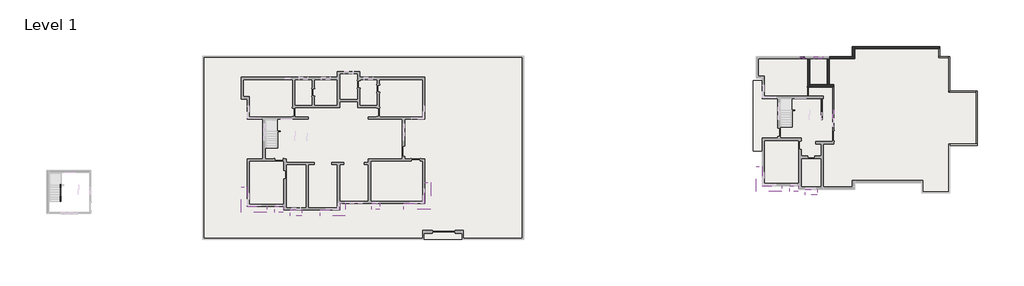
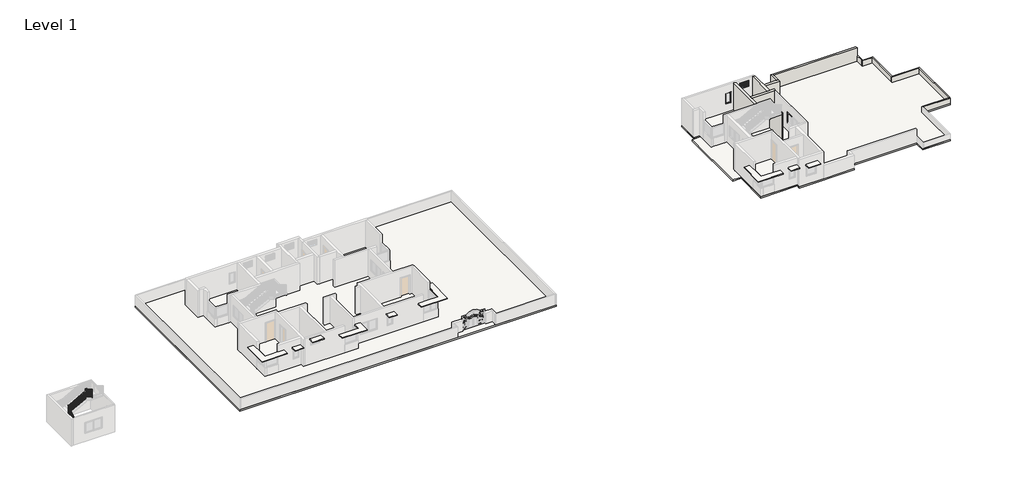
# One storey, part 4 of 9: 13 walls, 11 slabs, 6 members, 1 door, 1 railing, 1 window.
"""IFC4 building model written with IfcOpenShell, lengths in millimetres."""

from ifc_helpers import new_model, si_unit, frame, origin, origin_with_axes, place, context, project, spatial, polyline, outline, extrude, faceted_brep, transform, mapped, element, save
from components import single_flush_door_3_a90ba1ad, member_75074519, member_8d24a278, member_86d06fe4, window_a18e4be4

model = new_model("IFC4")

# Units and contexts
model_context = context("Model", 3, world=origin())
ifc_project = project(units=[si_unit("LENGTHUNIT", "METRE", prefix="MILLI")], contexts=[model_context])

# Site, building, storey
site = spatial("IfcSite", under=ifc_project)
building = spatial("IfcBuilding", under=site)
storey = spatial("IfcBuildingStorey", under=building, Name="Level 1", Elevation=0.0)

# Door
placement = place(None, origin())
single_flush_door_3_shape = single_flush_door_3_a90ba1ad(model_context)
element("IfcDoor", 1, ObjectType="Single-Flush : door 3'", at=placement, inside=storey, context=model_context, shape_type="MappedRepresentation", body=[
    mapped(single_flush_door_3_shape, transform((16302.8100959, 18368.9480703, 0.0), x_axis=(0.0, -1.0, 0.0), y_axis=(1.0, 0.0, 0.0), z_axis=(0.0, 0.0, 1.0))),
])

# Members
member_shape = member_75074519(model_context)
element("IfcMember", 2, ObjectType="Rectangular Mullion : 2.5\" x 5\" rectangular", at=placement, inside=storey, context=model_context, shape_type="MappedRepresentation", body=[
    mapped(member_shape, transform((15959.9100959, 21924.9480703, 914.4), x_axis=(1.0, 0.0, 0.0), y_axis=(0.0, -1.0, 0.0), z_axis=(0.0, 0.0, -1.0))),
])
element("IfcMember", 3, ObjectType="Rectangular Mullion : 2.5\" x 5\" rectangular", at=placement, inside=storey, context=model_context, shape_type="MappedRepresentation", body=[
    mapped(member_shape, transform((15350.3100959, 21924.9480703, 2133.6), x_axis=(-1.0, 0.0, 0.0), y_axis=(0.0, -1.0, 0.0), z_axis=(0.0, 0.0, 1.0))),
])
element("IfcMember", 4, ObjectType="Rectangular Mullion : 2.5\" x 5\" rectangular", at=placement, inside=storey, context=model_context, shape_type="MappedRepresentation", body=[
    mapped(member_shape, transform((18890.1839667, 16463.3540338, 914.4), x_axis=(0.0, 1.0, 0.0), y_axis=(1.0, 0.0, 0.0), z_axis=(0.0, 0.0, -1.0))),
])
member_2_shape = member_8d24a278(model_context)
element("IfcMember", 5, ObjectType="Rectangular Mullion : 2.5\" x 5\" rectangular", at=placement, inside=storey, context=model_context, shape_type="MappedRepresentation", body=[
    mapped(member_2_shape, transform((18890.1839667, 16399.8540338, 2133.6), x_axis=(0.0, 0.0, 1.0), y_axis=(1.0, 0.0, 0.0), z_axis=(0.0, 1.0, 0.0))),
])
member_3_shape = member_86d06fe4(model_context)
element("IfcMember", 6, ObjectType="Rectangular Mullion : 2.5\" x 5\" rectangular", at=placement, inside=storey, context=model_context, shape_type="MappedRepresentation", body=[
    mapped(member_3_shape, transform((15896.4100959, 21924.9480703, 2133.6), x_axis=(0.0, 0.0, 1.0), y_axis=(0.0, -1.0, 0.0), z_axis=(1.0, 0.0, 0.0))),
])
element("IfcMember", 7, ObjectType="Rectangular Mullion : 2.5\" x 5\" rectangular", at=placement, inside=storey, context=model_context, shape_type="MappedRepresentation", body=[
    mapped(member_3_shape, transform((15413.8100959, 21924.9480703, 914.4), x_axis=(0.0, 0.0, -1.0), y_axis=(0.0, -1.0, 0.0), z_axis=(-1.0, 0.0, 0.0))),
])

# Railing
element("IfcRailing", 8, ObjectType="Handrail - Rectangular", at=placement, inside=storey, context=model_context, shape_type="SolidModel", body=[
    faceted_brep([(-62595.4636189, 6754.3199577, 1059.5428571), (-62595.4636189, 6754.3199577, 1001.0339009), (-62544.6636189, 6754.3199577, 1001.0339009), (-62544.6636189, 6754.3199577, 1059.5428571), (-62595.4636189, 8456.1199577, 2032.0), (-62595.4636189, 8506.9199577, 2002.5196152), (-62544.6636189, 8506.9199577, 2002.5196152), (-62544.6636189, 8456.1199577, 2032.0), (-62595.4636189, 8456.1199577, 2261.3257143), (-62595.4636189, 8506.9199577, 2210.5257143), (-62544.6636189, 8506.9199577, 2210.5257143), (-62544.6636189, 8456.1199577, 2261.3257143), (-62595.4636189, 8583.1199577, 2261.3257143), (-62595.4636189, 8583.1199577, 2210.5257143), (-62544.6636189, 8532.3199577, 2210.5257143), (-62544.6636189, 8532.3199577, 2261.3257143), (-62468.4636189, 8583.1199577, 2261.3257143), (-62455.7636189, 8583.1199577, 2210.5257143), (-62455.7636189, 8532.3199577, 2210.5257143), (-62468.4636189, 8532.3199577, 2261.3257143), (-60715.8636189, 8583.1199577, 3196.0457143), (-60665.0636189, 8583.1199577, 3165.5657143), (-60665.0636189, 8532.3199577, 3165.5657143), (-60715.8636189, 8532.3199577, 3196.0457143), (-60715.8636189, 8583.1199577, 3425.3714286), (-60665.0636189, 8583.1199577, 3374.5714286), (-60665.0636189, 8532.3199577, 3374.5714286), (-60715.8636189, 8532.3199577, 3425.3714286), (-60588.8636189, 8583.1199577, 3425.3714286), (-60588.8636189, 8583.1199577, 3374.5714286), (-60639.6636189, 8532.3199577, 3374.5714286), (-60639.6636189, 8532.3199577, 3425.3714286), (-60588.8636189, 8456.1199577, 3425.3714286), (-60588.8636189, 8442.6292843, 3374.5714286), (-60639.6636189, 8442.6292843, 3374.5714286), (-60639.6636189, 8456.1199577, 3425.3714286), (-60588.8636189, 7516.3199577, 3962.4), (-60639.6636189, 7516.3199577, 3962.4), (-60639.6636189, 7516.3199577, 3903.8910438), (-60588.8636189, 7516.3199577, 3903.8910438)], [[[0, 1, 2, 3]], [[1, 0, 4, 5]], [[2, 1, 5, 6]], [[3, 2, 6, 7]], [[0, 3, 7, 4]], [[5, 4, 8, 9]], [[6, 5, 9, 10]], [[7, 6, 10, 11]], [[4, 7, 11, 8]], [[9, 8, 12, 13]], [[10, 9, 13, 14]], [[11, 10, 14, 15]], [[8, 11, 15, 12]], [[13, 12, 16, 17]], [[14, 13, 17, 18]], [[15, 14, 18, 19]], [[12, 15, 19, 16]], [[17, 16, 20, 21]], [[18, 17, 21, 22]], [[19, 18, 22, 23]], [[16, 19, 23, 20]], [[21, 20, 24, 25]], [[22, 21, 25, 26]], [[23, 22, 26, 27]], [[20, 23, 27, 24]], [[25, 24, 28, 29]], [[26, 25, 29, 30]], [[27, 26, 30, 31]], [[24, 27, 31, 28]], [[29, 28, 32, 33]], [[30, 29, 33, 34]], [[31, 30, 34, 35]], [[28, 31, 35, 32]], [[36, 37, 38, 39]], [[33, 32, 36, 39]], [[34, 33, 39, 38]], [[35, 34, 38, 37]], [[32, 35, 37, 36]]]),
    extrude(outline(polyline([(7532.1949577, 3894.8196152), (7551.2449577, 3883.9339009), (7551.2449577, 2902.8571429), (7532.1949577, 2902.8571429), (7532.1949577, 3894.8196152)])), frame((-60623.7886189, 0.0, 0.0), z_axis=(1.0, 0.0, 0.0), x_axis=(0.0, 1.0, 0.0)), (0.0, 0.0, 1.0), 19.05),
    extrude(outline(polyline([(7633.7949577, 3836.7624723), (7652.8449577, 3825.8767581), (7652.8449577, 2902.8571429), (7633.7949577, 2902.8571429), (7633.7949577, 3836.7624723)])), frame((-60623.7886189, 0.0, 0.0), z_axis=(1.0, 0.0, 0.0), x_axis=(0.0, 1.0, 0.0)), (0.0, 0.0, 1.0), 19.05),
    extrude(outline(polyline([(7735.3949577, 3778.7053295), (7754.4449577, 3767.8196152), (7754.4449577, 2902.8571429), (7735.3949577, 2902.8571429), (7735.3949577, 3778.7053295)])), frame((-60623.7886189, 0.0, 0.0), z_axis=(1.0, 0.0, 0.0), x_axis=(0.0, 1.0, 0.0)), (0.0, 0.0, 1.0), 19.05),
    extrude(outline(polyline([(7836.9949577, 3720.6481866), (7856.0449577, 3709.7624723), (7856.0449577, 2757.7142857), (7836.9949577, 2757.7142857), (7836.9949577, 3720.6481866)])), frame((-60623.7886189, 0.0, 0.0), z_axis=(1.0, 0.0, 0.0), x_axis=(0.0, 1.0, 0.0)), (0.0, 0.0, 1.0), 19.05),
    extrude(outline(polyline([(7938.5949577, 3662.5910438), (7957.6449577, 3651.7053295), (7957.6449577, 2757.7142857), (7938.5949577, 2757.7142857), (7938.5949577, 3662.5910438)])), frame((-60623.7886189, 0.0, 0.0), z_axis=(1.0, 0.0, 0.0), x_axis=(0.0, 1.0, 0.0)), (0.0, 0.0, 1.0), 19.05),
    extrude(outline(polyline([(8040.1949577, 3604.5339009), (8059.2449577, 3593.6481866), (8059.2449577, 2612.5714286), (8040.1949577, 2612.5714286), (8040.1949577, 3604.5339009)])), frame((-60623.7886189, 0.0, 0.0), z_axis=(1.0, 0.0, 0.0), x_axis=(0.0, 1.0, 0.0)), (0.0, 0.0, 1.0), 19.05),
    extrude(outline(polyline([(8141.7949577, 3546.4767581), (8160.8449577, 3535.5910438), (8160.8449577, 2612.5714286), (8141.7949577, 2612.5714286), (8141.7949577, 3546.4767581)])), frame((-60623.7886189, 0.0, 0.0), z_axis=(1.0, 0.0, 0.0), x_axis=(0.0, 1.0, 0.0)), (0.0, 0.0, 1.0), 19.05),
    extrude(outline(polyline([(8243.3949577, 3488.4196152), (8262.4449577, 3477.5339009), (8262.4449577, 2612.5714286), (8243.3949577, 2612.5714286), (8243.3949577, 3488.4196152)])), frame((-60623.7886189, 0.0, 0.0), z_axis=(1.0, 0.0, 0.0), x_axis=(0.0, 1.0, 0.0)), (0.0, 0.0, 1.0), 19.05),
    extrude(outline(polyline([(8344.9949577, 3430.3624723), (8364.0449577, 3419.4767581), (8364.0449577, 2467.4285714), (8344.9949577, 2467.4285714), (8344.9949577, 3430.3624723)])), frame((-60623.7886189, 0.0, 0.0), z_axis=(1.0, 0.0, 0.0), x_axis=(0.0, 1.0, 0.0)), (0.0, 0.0, 1.0), 19.05),
    extrude(outline(polyline([(8446.5949577, 3372.3053295), (8465.6449577, 3361.4196152), (8465.6449577, 2467.4285714), (8446.5949577, 2467.4285714), (8446.5949577, 3372.3053295)])), frame((-60623.7886189, 0.0, 0.0), z_axis=(1.0, 0.0, 0.0), x_axis=(0.0, 1.0, 0.0)), (0.0, 0.0, 1.0), 19.05),
    extrude(outline(polyline([(-60649.1886189, 8548.1949577), (-60649.1886189, 8567.2449577), (-60630.1386189, 8567.2449577), (-60630.1386189, 8548.1949577), (-60649.1886189, 8548.1949577)])), frame((0.0, 0.0, 2322.2857143), z_axis=(0.0, 0.0, 1.0), x_axis=(1.0, 0.0, 0.0)), (0.0, 0.0, 1.0), 1052.2857143),
    extrude(outline(polyline([(3130.0057143, -60731.7386189), (3119.8457143, -60750.7886189), (2177.1428571, -60750.7886189), (2177.1428571, -60731.7386189), (3130.0057143, -60731.7386189)])), frame((0.0, 8548.1949577, 0.0), z_axis=(0.0, 1.0, 0.0), x_axis=(0.0, 0.0, 1.0)), (0.0, 0.0, 1.0), 19.05),
    extrude(outline(polyline([(3075.8190476, -60833.3386189), (3065.6590476, -60852.3886189), (2177.1428571, -60852.3886189), (2177.1428571, -60833.3386189), (3075.8190476, -60833.3386189)])), frame((0.0, 8548.1949577, 0.0), z_axis=(0.0, 1.0, 0.0), x_axis=(0.0, 0.0, 1.0)), (0.0, 0.0, 1.0), 19.05),
    extrude(outline(polyline([(3021.632381, -60934.9386189), (3011.472381, -60953.9886189), (2032.0, -60953.9886189), (2032.0, -60934.9386189), (3021.632381, -60934.9386189)])), frame((0.0, 8548.1949577, 0.0), z_axis=(0.0, 1.0, 0.0), x_axis=(0.0, 0.0, 1.0)), (0.0, 0.0, 1.0), 19.05),
    extrude(outline(polyline([(2967.4457143, -61036.5386189), (2957.2857143, -61055.5886189), (2032.0, -61055.5886189), (2032.0, -61036.5386189), (2967.4457143, -61036.5386189)])), frame((0.0, 8548.1949577, 0.0), z_axis=(0.0, 1.0, 0.0), x_axis=(0.0, 0.0, 1.0)), (0.0, 0.0, 1.0), 19.05),
    extrude(outline(polyline([(2913.2590476, -61138.1386189), (2903.0990476, -61157.1886189), (2032.0, -61157.1886189), (2032.0, -61138.1386189), (2913.2590476, -61138.1386189)])), frame((0.0, 8548.1949577, 0.0), z_axis=(0.0, 1.0, 0.0), x_axis=(0.0, 0.0, 1.0)), (0.0, 0.0, 1.0), 19.05),
    extrude(outline(polyline([(2859.072381, -61239.7386189), (2848.912381, -61258.7886189), (1886.8571429, -61258.7886189), (1886.8571429, -61239.7386189), (2859.072381, -61239.7386189)])), frame((0.0, 8548.1949577, 0.0), z_axis=(0.0, 1.0, 0.0), x_axis=(0.0, 0.0, 1.0)), (0.0, 0.0, 1.0), 19.05),
    extrude(outline(polyline([(2804.8857143, -61341.3386189), (2794.7257143, -61360.3886189), (1886.8571429, -61360.3886189), (1886.8571429, -61341.3386189), (2804.8857143, -61341.3386189)])), frame((0.0, 8548.1949577, 0.0), z_axis=(0.0, 1.0, 0.0), x_axis=(0.0, 0.0, 1.0)), (0.0, 0.0, 1.0), 19.05),
    extrude(outline(polyline([(2750.6990476, -61442.9386189), (2740.5390476, -61461.9886189), (1886.8571429, -61461.9886189), (1886.8571429, -61442.9386189), (2750.6990476, -61442.9386189)])), frame((0.0, 8548.1949577, 0.0), z_axis=(0.0, 1.0, 0.0), x_axis=(0.0, 0.0, 1.0)), (0.0, 0.0, 1.0), 19.05),
    extrude(outline(polyline([(2696.512381, -61544.5386189), (2686.352381, -61563.5886189), (1741.7142857, -61563.5886189), (1741.7142857, -61544.5386189), (2696.512381, -61544.5386189)])), frame((0.0, 8548.1949577, 0.0), z_axis=(0.0, 1.0, 0.0), x_axis=(0.0, 0.0, 1.0)), (0.0, 0.0, 1.0), 19.05),
    extrude(outline(polyline([(2642.3257143, -61646.1386189), (2632.1657143, -61665.1886189), (1741.7142857, -61665.1886189), (1741.7142857, -61646.1386189), (2642.3257143, -61646.1386189)])), frame((0.0, 8548.1949577, 0.0), z_axis=(0.0, 1.0, 0.0), x_axis=(0.0, 0.0, 1.0)), (0.0, 0.0, 1.0), 19.05),
    extrude(outline(polyline([(2588.1390476, -61747.7386189), (2577.9790476, -61766.7886189), (1596.5714286, -61766.7886189), (1596.5714286, -61747.7386189), (2588.1390476, -61747.7386189)])), frame((0.0, 8548.1949577, 0.0), z_axis=(0.0, 1.0, 0.0), x_axis=(0.0, 0.0, 1.0)), (0.0, 0.0, 1.0), 19.05),
    extrude(outline(polyline([(2533.952381, -61849.3386189), (2523.792381, -61868.3886189), (1596.5714286, -61868.3886189), (1596.5714286, -61849.3386189), (2533.952381, -61849.3386189)])), frame((0.0, 8548.1949577, 0.0), z_axis=(0.0, 1.0, 0.0), x_axis=(0.0, 0.0, 1.0)), (0.0, 0.0, 1.0), 19.05),
    extrude(outline(polyline([(2479.7657143, -61950.9386189), (2469.6057143, -61969.9886189), (1596.5714286, -61969.9886189), (1596.5714286, -61950.9386189), (2479.7657143, -61950.9386189)])), frame((0.0, 8548.1949577, 0.0), z_axis=(0.0, 1.0, 0.0), x_axis=(0.0, 0.0, 1.0)), (0.0, 0.0, 1.0), 19.05),
    extrude(outline(polyline([(2425.5790476, -62052.5386189), (2415.4190476, -62071.5886189), (1451.4285714, -62071.5886189), (1451.4285714, -62052.5386189), (2425.5790476, -62052.5386189)])), frame((0.0, 8548.1949577, 0.0), z_axis=(0.0, 1.0, 0.0), x_axis=(0.0, 0.0, 1.0)), (0.0, 0.0, 1.0), 19.05),
    extrude(outline(polyline([(2371.392381, -62154.1386189), (2361.232381, -62173.1886189), (1451.4285714, -62173.1886189), (1451.4285714, -62154.1386189), (2371.392381, -62154.1386189)])), frame((0.0, 8548.1949577, 0.0), z_axis=(0.0, 1.0, 0.0), x_axis=(0.0, 0.0, 1.0)), (0.0, 0.0, 1.0), 19.05),
    extrude(outline(polyline([(2317.2057143, -62255.7386189), (2307.0457143, -62274.7886189), (1451.4285714, -62274.7886189), (1451.4285714, -62255.7386189), (2317.2057143, -62255.7386189)])), frame((0.0, 8548.1949577, 0.0), z_axis=(0.0, 1.0, 0.0), x_axis=(0.0, 0.0, 1.0)), (0.0, 0.0, 1.0), 19.05),
    extrude(outline(polyline([(2263.0190476, -62357.3386189), (2252.8590476, -62376.3886189), (1306.2857143, -62376.3886189), (1306.2857143, -62357.3386189), (2263.0190476, -62357.3386189)])), frame((0.0, 8548.1949577, 0.0), z_axis=(0.0, 1.0, 0.0), x_axis=(0.0, 0.0, 1.0)), (0.0, 0.0, 1.0), 19.05),
    extrude(outline(polyline([(2208.832381, -62458.9386189), (2198.672381, -62477.9886189), (1306.2857143, -62477.9886189), (1306.2857143, -62458.9386189), (2208.832381, -62458.9386189)])), frame((0.0, 8548.1949577, 0.0), z_axis=(0.0, 1.0, 0.0), x_axis=(0.0, 0.0, 1.0)), (0.0, 0.0, 1.0), 19.05),
    extrude(outline(polyline([(-62560.5386189, 8471.9949577), (-62579.5886189, 8471.9949577), (-62579.5886189, 8491.0449577), (-62560.5386189, 8491.0449577), (-62560.5386189, 8471.9949577)])), frame((0.0, 0.0, 1016.0), z_axis=(0.0, 0.0, 1.0), x_axis=(1.0, 0.0, 0.0)), (0.0, 0.0, 1.0), 1194.5257143),
    extrude(outline(polyline([(8370.3949577, 1924.5053295), (8389.4449577, 1935.3910438), (8389.4449577, 1016.0), (8370.3949577, 1016.0), (8370.3949577, 1924.5053295)])), frame((-62579.5886189, 0.0, 0.0), z_axis=(1.0, 0.0, 0.0), x_axis=(0.0, 1.0, 0.0)), (0.0, 0.0, 1.0), 19.05),
    extrude(outline(polyline([(8268.7949577, 1866.4481866), (8287.8449577, 1877.3339009), (8287.8449577, 1016.0), (8268.7949577, 1016.0), (8268.7949577, 1866.4481866)])), frame((-62579.5886189, 0.0, 0.0), z_axis=(1.0, 0.0, 0.0), x_axis=(0.0, 1.0, 0.0)), (0.0, 0.0, 1.0), 19.05),
    extrude(outline(polyline([(8167.1949577, 1808.3910438), (8186.2449577, 1819.2767581), (8186.2449577, 870.8571429), (8167.1949577, 870.8571429), (8167.1949577, 1808.3910438)])), frame((-62579.5886189, 0.0, 0.0), z_axis=(1.0, 0.0, 0.0), x_axis=(0.0, 1.0, 0.0)), (0.0, 0.0, 1.0), 19.05),
    extrude(outline(polyline([(8065.5949577, 1750.3339009), (8084.6449577, 1761.2196152), (8084.6449577, 870.8571429), (8065.5949577, 870.8571429), (8065.5949577, 1750.3339009)])), frame((-62579.5886189, 0.0, 0.0), z_axis=(1.0, 0.0, 0.0), x_axis=(0.0, 1.0, 0.0)), (0.0, 0.0, 1.0), 19.05),
    extrude(outline(polyline([(7963.9949577, 1692.2767581), (7983.0449577, 1703.1624723), (7983.0449577, 725.7142857), (7963.9949577, 725.7142857), (7963.9949577, 1692.2767581)])), frame((-62579.5886189, 0.0, 0.0), z_axis=(1.0, 0.0, 0.0), x_axis=(0.0, 1.0, 0.0)), (0.0, 0.0, 1.0), 19.05),
    extrude(outline(polyline([(7862.3949577, 1634.2196152), (7881.4449577, 1645.1053295), (7881.4449577, 725.7142857), (7862.3949577, 725.7142857), (7862.3949577, 1634.2196152)])), frame((-62579.5886189, 0.0, 0.0), z_axis=(1.0, 0.0, 0.0), x_axis=(0.0, 1.0, 0.0)), (0.0, 0.0, 1.0), 19.05),
    extrude(outline(polyline([(7760.7949577, 1576.1624723), (7779.8449577, 1587.0481866), (7779.8449577, 725.7142857), (7760.7949577, 725.7142857), (7760.7949577, 1576.1624723)])), frame((-62579.5886189, 0.0, 0.0), z_axis=(1.0, 0.0, 0.0), x_axis=(0.0, 1.0, 0.0)), (0.0, 0.0, 1.0), 19.05),
    extrude(outline(polyline([(7659.1949577, 1518.1053295), (7678.2449577, 1528.9910438), (7678.2449577, 580.5714286), (7659.1949577, 580.5714286), (7659.1949577, 1518.1053295)])), frame((-62579.5886189, 0.0, 0.0), z_axis=(1.0, 0.0, 0.0), x_axis=(0.0, 1.0, 0.0)), (0.0, 0.0, 1.0), 19.05),
    extrude(outline(polyline([(7557.5949577, 1460.0481866), (7576.6449577, 1470.9339009), (7576.6449577, 580.5714286), (7557.5949577, 580.5714286), (7557.5949577, 1460.0481866)])), frame((-62579.5886189, 0.0, 0.0), z_axis=(1.0, 0.0, 0.0), x_axis=(0.0, 1.0, 0.0)), (0.0, 0.0, 1.0), 19.05),
    extrude(outline(polyline([(7455.9949577, 1401.9910438), (7475.0449577, 1412.8767581), (7475.0449577, 435.4285714), (7455.9949577, 435.4285714), (7455.9949577, 1401.9910438)])), frame((-62579.5886189, 0.0, 0.0), z_axis=(1.0, 0.0, 0.0), x_axis=(0.0, 1.0, 0.0)), (0.0, 0.0, 1.0), 19.05),
    extrude(outline(polyline([(7354.3949577, 1343.9339009), (7373.4449577, 1354.8196152), (7373.4449577, 435.4285714), (7354.3949577, 435.4285714), (7354.3949577, 1343.9339009)])), frame((-62579.5886189, 0.0, 0.0), z_axis=(1.0, 0.0, 0.0), x_axis=(0.0, 1.0, 0.0)), (0.0, 0.0, 1.0), 19.05),
    extrude(outline(polyline([(7252.7949577, 1285.8767581), (7271.8449577, 1296.7624723), (7271.8449577, 435.4285714), (7252.7949577, 435.4285714), (7252.7949577, 1285.8767581)])), frame((-62579.5886189, 0.0, 0.0), z_axis=(1.0, 0.0, 0.0), x_axis=(0.0, 1.0, 0.0)), (0.0, 0.0, 1.0), 19.05),
    extrude(outline(polyline([(7151.1949577, 1227.8196152), (7170.2449577, 1238.7053295), (7170.2449577, 290.2857143), (7151.1949577, 290.2857143), (7151.1949577, 1227.8196152)])), frame((-62579.5886189, 0.0, 0.0), z_axis=(1.0, 0.0, 0.0), x_axis=(0.0, 1.0, 0.0)), (0.0, 0.0, 1.0), 19.05),
    extrude(outline(polyline([(7049.5949577, 1169.7624723), (7068.6449577, 1180.6481866), (7068.6449577, 290.2857143), (7049.5949577, 290.2857143), (7049.5949577, 1169.7624723)])), frame((-62579.5886189, 0.0, 0.0), z_axis=(1.0, 0.0, 0.0), x_axis=(0.0, 1.0, 0.0)), (0.0, 0.0, 1.0), 19.05),
    extrude(outline(polyline([(6947.9949577, 1111.7053295), (6967.0449577, 1122.5910438), (6967.0449577, 145.1428571), (6947.9949577, 145.1428571), (6947.9949577, 1111.7053295)])), frame((-62579.5886189, 0.0, 0.0), z_axis=(1.0, 0.0, 0.0), x_axis=(0.0, 1.0, 0.0)), (0.0, 0.0, 1.0), 19.05),
    extrude(outline(polyline([(6846.3949577, 1053.6481866), (6865.4449577, 1064.5339009), (6865.4449577, 145.1428571), (6846.3949577, 145.1428571), (6846.3949577, 1053.6481866)])), frame((-62579.5886189, 0.0, 0.0), z_axis=(1.0, 0.0, 0.0), x_axis=(0.0, 1.0, 0.0)), (0.0, 0.0, 1.0), 19.05),
    extrude(outline(polyline([(-60623.7886189, 8548.1949577), (-60623.7886189, 8567.2449577), (-60604.7386189, 8567.2449577), (-60604.7386189, 8548.1949577), (-60623.7886189, 8548.1949577)])), frame((0.0, 0.0, 2322.2857143), z_axis=(0.0, 0.0, 1.0), x_axis=(1.0, 0.0, 0.0)), (0.0, 0.0, 1.0), 1052.2857143),
    extrude(outline(polyline([(-62560.5386189, 8548.1949577), (-62579.5886189, 8548.1949577), (-62579.5886189, 8567.2449577), (-62560.5386189, 8567.2449577), (-62560.5386189, 8548.1949577)])), frame((0.0, 0.0, 1161.1428571), z_axis=(0.0, 0.0, 1.0), x_axis=(1.0, 0.0, 0.0)), (0.0, 0.0, 1.0), 1049.3828571),
    extrude(outline(polyline([(7516.3199577, 3903.8910438), (7535.3699577, 3893.0053295), (7535.3699577, 2902.8571429), (7516.3199577, 2902.8571429), (7516.3199577, 3903.8910438)])), frame((-60623.7886189, 0.0, 0.0), z_axis=(1.0, 0.0, 0.0), x_axis=(0.0, 1.0, 0.0)), (0.0, 0.0, 1.0), 19.05),
    extrude(outline(polyline([(6754.3199577, 1001.0339009), (6773.3699577, 1011.9196152), (6773.3699577, 145.1428571), (6754.3199577, 145.1428571), (6754.3199577, 1001.0339009)])), frame((-62579.5886189, 0.0, 0.0), z_axis=(1.0, 0.0, 0.0), x_axis=(0.0, 1.0, 0.0)), (0.0, 0.0, 1.0), 19.05),
])

# Slabs
element("IfcSlab", 9, ObjectType="FLOOR 6\"", at=placement, inside=storey, context=model_context, shape_type="SweptSolid", body=[
    extrude(outline(polyline([(-13760.2146233, 22130.8624892), (-13760.2146233, 2776.0624892), (-47593.0146233, 2776.0624892), (-47593.0146233, 22130.8624892), (-13760.2146233, 22130.8624892)])), frame((0.0, 0.0, -152.4), z_axis=(0.0, 0.0, 1.0), x_axis=(1.0, 0.0, 0.0)), (0.0, 0.0, 1.0), 152.4),
])
element("IfcSlab", 10, ObjectType="FLOOR 6\"", at=placement, inside=storey, context=model_context, shape_type="SweptSolid", body=[
    extrude(outline(polyline([(10473.5100959, 19545.7642649), (11387.9100959, 19545.7642649), (11387.9100959, 19778.6480703), (10778.3100959, 19778.6480703), (10778.3100959, 22064.6480703), (20912.4092023, 22064.6480703), (20912.4092023, 23131.4480703), (30133.1100959, 23131.4480703), (30133.1100959, 22064.6480703), (31199.9100959, 22064.6480703), (31199.9100959, 18407.0480703), (34095.5100959, 18407.0480703), (34095.5100959, 12692.0480703), (31199.9100959, 12692.0480703), (31199.9100959, 7662.8480703), (28228.1100959, 7662.8480703), (28228.1100959, 8729.6480703), (21141.5100959, 8729.6480703), (21141.5100959, 8043.769664), (15274.1100959, 8043.769664), (15274.1100959, 8424.8480703), (11387.9100959, 8424.8480703), (11387.9100959, 12082.4480703), (10473.5100959, 12082.4480703), (10473.5100959, 19545.7642649)])), frame((0.0, 0.0, -152.4), z_axis=(0.0, 0.0, 1.0), x_axis=(1.0, 0.0, 0.0)), (0.0, 0.0, 1.0), 152.4),
])
element("IfcSlab", 11, ObjectType="Generic - 12\"", at=placement, inside=storey, context=model_context, shape_type="SweptSolid", body=[
    extrude(outline(polyline([(-35210.5146233, 5252.484083), (-35210.5146233, 5862.084083), (-33153.1146233, 5862.084083), (-33153.1146233, 6547.9624892), (-32543.5146233, 6547.9624892), (-32543.5146233, 5252.484083), (-35210.5146233, 5252.484083)])), frame((0.0, 0.0, 2209.8), z_axis=(0.0, 0.0, 1.0), x_axis=(1.0, 0.0, 0.0)), (0.0, 0.0, 1.0), 76.2),
])
element("IfcSlab", 12, ObjectType="Generic - 12\"", at=placement, inside=storey, context=model_context, shape_type="SweptSolid", body=[
    extrude(outline(polyline([(-29762.1467796, 5938.3624892), (-29762.1467796, 6547.9624892), (-28925.793098, 6547.9624892), (-28925.793098, 5938.3624892), (-29762.1467796, 5938.3624892)])), frame((0.0, 0.0, 2209.8), z_axis=(0.0, 0.0, 1.0), x_axis=(1.0, 0.0, 0.0)), (0.0, 0.0, 1.0), 76.2),
])
element("IfcSlab", 13, ObjectType="Generic - 12\"", at=placement, inside=storey, context=model_context, shape_type="SweptSolid", body=[
    extrude(outline(polyline([(-26371.3146233, 5938.3624892), (-26371.3146233, 6547.9624892), (-24161.5146233, 6547.9624892), (-24161.5146233, 8757.7624892), (-23551.9146233, 8757.7624892), (-23551.9146233, 5938.3624892), (-26371.3146233, 5938.3624892)])), frame((0.0, 0.0, 2209.8), z_axis=(0.0, 0.0, 1.0), x_axis=(1.0, 0.0, 0.0)), (0.0, 0.0, 1.0), 76.2),
])
element("IfcSlab", 14, ObjectType="Generic - 12\"", at=placement, inside=storey, context=model_context, shape_type="SweptSolid", body=[
    extrude(outline(polyline([(-43516.3146234, 8300.5624892), (-42906.7146233, 8300.5624892), (-42906.7146233, 6243.1624892), (-40849.3146233, 6243.1624892), (-40849.3146233, 5633.5624892), (-43516.3146234, 5633.5624892), (-43516.3146234, 8300.5624892)])), frame((0.0, 0.0, 2209.8), z_axis=(0.0, 0.0, 1.0), x_axis=(1.0, 0.0, 0.0)), (0.0, 0.0, 1.0), 76.2),
])
element("IfcSlab", 15, ObjectType="Generic - 12\"", at=placement, inside=storey, context=model_context, shape_type="SweptSolid", body=[
    extrude(outline(polyline([(-40011.1146233, 5633.5624892), (-40011.1146233, 6243.1624892), (-39096.7146233, 6243.1624892), (-39096.7146233, 5633.5624892), (-40011.1146233, 5633.5624892)])), frame((0.0, 0.0, 2209.8), z_axis=(0.0, 0.0, 1.0), x_axis=(1.0, 0.0, 0.0)), (0.0, 0.0, 1.0), 76.2),
])
element("IfcSlab", 16, ObjectType="Generic - 12\"", at=placement, inside=storey, context=model_context, shape_type="SweptSolid", body=[
    extrude(outline(polyline([(-38334.7146233, 5252.484083), (-38334.7146233, 5862.084083), (-37115.5146233, 5862.084083), (-37115.5146233, 5252.484083), (-38334.7146233, 5252.484083)])), frame((0.0, 0.0, 2819.4), z_axis=(0.0, 0.0, 1.0), x_axis=(1.0, 0.0, 0.0)), (0.0, 0.0, 1.0), 76.2),
])
element("IfcSlab", 17, ObjectType="Generic - 12\"", at=placement, inside=storey, context=model_context, shape_type="SweptSolid", body=[
    extrude(outline(polyline([(10778.3100959, 10482.2480703), (11387.9100959, 10482.2480703), (11387.9100959, 8424.8480703), (13445.3100959, 8424.8480703), (13445.3100959, 7815.2480703), (10778.3100959, 7815.2480703), (10778.3100959, 10482.2480703)])), frame((0.0, 0.0, 2209.8), z_axis=(0.0, 0.0, 1.0), x_axis=(1.0, 0.0, 0.0)), (0.0, 0.0, 1.0), 76.2),
])
element("IfcSlab", 18, ObjectType="Generic - 12\"", at=placement, inside=storey, context=model_context, shape_type="SweptSolid", body=[
    extrude(outline(polyline([(14283.5100959, 7815.2480703), (14283.5100959, 8424.8480703), (15197.9100959, 8424.8480703), (15197.9100959, 7815.2480703), (14283.5100959, 7815.2480703)])), frame((0.0, 0.0, 2209.8), z_axis=(0.0, 0.0, 1.0), x_axis=(1.0, 0.0, 0.0)), (0.0, 0.0, 1.0), 76.2),
])
element("IfcSlab", 19, ObjectType="Generic - 12\"", at=placement, inside=storey, context=model_context, shape_type="SweptSolid", body=[
    extrude(outline(polyline([(15921.8100959, 7434.169664), (15921.8100959, 8043.769664), (17217.2100959, 8043.769664), (17217.2100959, 7434.169664), (15921.8100959, 7434.169664)])), frame((0.0, 0.0, 2209.8), z_axis=(0.0, 0.0, 1.0), x_axis=(1.0, 0.0, 0.0)), (0.0, 0.0, 1.0), 76.2),
])

# Walls
element("IfcWall", 20, at=placement, inside=storey, context=model_context, shape_type="Brep", body=[
    faceted_brep([(18474.5100959, 21836.0480703, 0.0), (21141.0092023, 21836.0480703, 0.0), (21141.0092023, 21836.0480703, 1524.0), (18474.5100959, 21836.0480703, 1524.0), (18474.5100959, 22064.6480703, 0.0), (18474.5100959, 22064.6480703, 1524.0), (20912.4092023, 22064.6480703, 1524.0), (21141.0092023, 22064.6480703, 1524.0), (21141.0092023, 22064.6480703, 0.0), (20912.4092023, 22064.6480703, 0.0)], [[[0, 1, 2, 3]], [[4, 5, 6, 7, 8, 9]], [[1, 0, 4, 9, 8]], [[3, 2, 7, 6, 5]], [[0, 3, 5, 4]], [[2, 1, 8, 7]]]),
])
element("IfcWall", 21, at=placement, inside=storey, context=model_context, shape_type="Brep", body=[
    faceted_brep([(21141.0092023, 22064.6480703, 0.0), (21141.0092023, 22902.8480703, 0.0), (21141.0092023, 23131.4480703, 0.0), (21141.0092023, 23131.4480703, 1524.0), (21141.0092023, 22902.8480703, 1524.0), (21141.0092023, 22064.6480703, 1524.0), (20912.4092023, 22064.6480703, 0.0), (20912.4092023, 22064.6480703, 1524.0), (20912.4092023, 23131.4480703, 1524.0), (20912.4092023, 23131.4480703, 0.0)], [[[0, 1, 2, 3, 4, 5]], [[6, 7, 8, 9]], [[2, 1, 0, 6, 9]], [[5, 4, 3, 8, 7]], [[0, 5, 7, 6]], [[3, 2, 9, 8]]]),
])
element("IfcWall", 22, at=placement, inside=storey, context=model_context, shape_type="Brep", body=[
    faceted_brep([(21141.0092023, 22902.8480703, 0.0), (30018.8100959, 22902.8480703, 0.0), (30018.8100959, 22902.8480703, 1524.0), (21141.0092023, 22902.8480703, 1524.0), (21141.0092023, 23131.4480703, 0.0), (21141.0092023, 23131.4480703, 1524.0), (30018.8100959, 23131.4480703, 1524.0), (30018.8100959, 23131.4480703, 609.6), (30018.8100959, 23131.4480703, 0.0)], [[[0, 1, 2, 3]], [[4, 5, 6, 7, 8]], [[1, 0, 4, 8]], [[3, 2, 6, 5]], [[0, 3, 5, 4]], [[2, 1, 8, 7, 6]]]),
])
element("IfcWall", 23, at=placement, inside=storey, context=model_context, shape_type="Brep", body=[
    faceted_brep([(31199.9100959, 12692.0480703, 0.0), (34095.5100959, 12692.0480703, 0.0), (34095.5100959, 12692.0480703, 609.6), (31199.9100959, 12692.0480703, 609.6), (31199.9100959, 12806.3480703, 0.0), (31199.9100959, 12806.3480703, 609.6), (33981.2100959, 12806.3480703, 609.6), (34095.5100959, 12806.3480703, 609.6), (34095.5100959, 12806.3480703, 0.0), (33981.2100959, 12806.3480703, 0.0)], [[[0, 1, 2, 3]], [[4, 5, 6, 7, 8, 9]], [[1, 0, 4, 9, 8]], [[3, 2, 7, 6, 5]], [[0, 3, 5, 4]], [[2, 1, 8, 7]]]),
])
element("IfcWall", 24, at=placement, inside=storey, context=model_context, shape_type="Brep", body=[
    faceted_brep([(34095.5100959, 12806.3480703, 0.0), (34095.5100959, 18407.0480703, 0.0), (34095.5100959, 18407.0480703, 609.6), (34095.5100959, 12806.3480703, 609.6), (33981.2100959, 12806.3480703, 0.0), (33981.2100959, 12806.3480703, 609.6), (33981.2100959, 18292.7480703, 609.6), (33981.2100959, 18407.0480703, 609.6), (33981.2100959, 18407.0480703, 0.0), (33981.2100959, 18292.7480703, 0.0)], [[[0, 1, 2, 3]], [[4, 5, 6, 7, 8, 9]], [[1, 0, 4, 9, 8]], [[3, 2, 7, 6, 5]], [[0, 3, 5, 4]], [[2, 1, 8, 7]]]),
])
element("IfcWall", 25, at=placement, inside=storey, context=model_context, shape_type="Brep", body=[
    faceted_brep([(33981.2100959, 18407.0480703, 0.0), (31199.9100959, 18407.0480703, 0.0), (31085.6100959, 18407.0480703, 0.0), (31085.6100959, 18407.0480703, 609.6), (31199.9100959, 18407.0480703, 609.6), (33981.2100959, 18407.0480703, 609.6), (33981.2100959, 18292.7480703, 0.0), (33981.2100959, 18292.7480703, 609.6), (31085.6100959, 18292.7480703, 609.6), (31085.6100959, 18292.7480703, 0.0)], [[[0, 1, 2, 3, 4, 5]], [[6, 7, 8, 9]], [[2, 1, 0, 6, 9]], [[5, 4, 3, 8, 7]], [[0, 5, 7, 6]], [[3, 2, 9, 8]]]),
])
element("IfcWall", 26, at=placement, inside=storey, context=model_context, shape_type="Brep", body=[
    faceted_brep([(31199.9100959, 18407.0480703, 0.0), (31199.9100959, 22064.6480703, 0.0), (31199.9100959, 22064.6480703, 609.6), (31199.9100959, 18407.0480703, 609.6), (31085.6100959, 18407.0480703, 0.0), (31085.6100959, 18407.0480703, 609.6), (31085.6100959, 21950.3480703, 609.6), (31085.6100959, 22064.6480703, 609.6), (31085.6100959, 22064.6480703, 0.0), (31085.6100959, 21950.3480703, 0.0)], [[[0, 1, 2, 3]], [[4, 5, 6, 7, 8, 9]], [[1, 0, 4, 9, 8]], [[3, 2, 7, 6, 5]], [[0, 3, 5, 4]], [[2, 1, 8, 7]]]),
])
element("IfcWall", 27, at=placement, inside=storey, context=model_context, shape_type="Brep", body=[
    faceted_brep([(31085.6100959, 22064.6480703, 0.0), (30133.1100959, 22064.6480703, 0.0), (30018.8100959, 22064.6480703, 0.0), (30018.8100959, 22064.6480703, 609.6), (30133.1100959, 22064.6480703, 609.6), (31085.6100959, 22064.6480703, 609.6), (31085.6100959, 21950.3480703, 0.0), (31085.6100959, 21950.3480703, 609.6), (30018.8100959, 21950.3480703, 609.6), (30018.8100959, 21950.3480703, 0.0)], [[[0, 1, 2, 3, 4, 5]], [[6, 7, 8, 9]], [[2, 1, 0, 6, 9]], [[5, 4, 3, 8, 7]], [[0, 5, 7, 6]], [[3, 2, 9, 8]]]),
])
element("IfcWall", 28, at=placement, inside=storey, context=model_context, shape_type="Brep", body=[
    faceted_brep([(30133.1100959, 22064.6480703, 0.0), (30133.1100959, 23131.4480703, 0.0), (30133.1100959, 23131.4480703, 609.6), (30133.1100959, 22064.6480703, 609.6), (30018.8100959, 22064.6480703, 0.0), (30018.8100959, 22064.6480703, 609.6), (30018.8100959, 23131.4480703, 609.6), (30018.8100959, 23131.4480703, 0.0), (30018.8100959, 22902.8480703, 0.0)], [[[0, 1, 2, 3]], [[4, 5, 6, 7, 8]], [[1, 0, 4, 8, 7]], [[3, 2, 6, 5]], [[0, 3, 5, 4]], [[2, 1, 7, 6]]]),
])
element("IfcWall", 29, ObjectType="Generic - 5\"", at=placement, inside=storey, context=model_context, shape_type="SweptSolid", body=[
    extrude(outline(polyline([(17636.3100959, 15409.8480703), (17636.3100959, 17645.0480703), (17750.6100959, 17645.0480703), (17750.6100959, 15409.8480703), (17636.3100959, 15409.8480703)])), origin_with_axes(), (0.0, 0.0, 1.0), 3048.0),
])
element("IfcWall", 30, ObjectType="WALL 9\"", at=placement, inside=storey, context=model_context, shape_type="SweptSolid", body=[
    extrude(outline(polyline([(18245.9100959, 19092.8480703), (18245.9100959, 21836.0480703), (18474.5100959, 21836.0480703), (18474.5100959, 19092.8480703), (18245.9100959, 19092.8480703)])), origin_with_axes(), (0.0, 0.0, 1.0), 3048.0),
])
element("IfcWall", 31, ObjectType="WALL 9\"", at=placement, inside=storey, context=model_context, shape_type="Brep", body=[
    faceted_brep([(16188.5100959, 17911.7480703, 2133.6), (16188.5100959, 17911.7480703, 0.0), (16188.5100959, 17873.6480703, 0.0), (16188.5100959, 17873.6480703, 3048.0), (16188.5100959, 21836.0480703, 3048.0), (16188.5100959, 21836.0480703, 0.0), (16188.5100959, 18826.1480703, 0.0), (16188.5100959, 18826.1480703, 2133.6), (16417.1100959, 17873.6480703, 0.0), (16417.1100959, 17911.7480703, 0.0), (16417.1100959, 17911.7480703, 2133.6), (16417.1100959, 18826.1480703, 2133.6), (16417.1100959, 18826.1480703, 0.0), (16417.1100959, 18864.2480703, 0.0), (16417.1100959, 19092.8480703, 0.0), (16417.1100959, 21836.0480703, 0.0), (16417.1100959, 21836.0480703, 3048.0), (16417.1100959, 19092.8480703, 3048.0), (16417.1100959, 18864.2480703, 3048.0), (16417.1100959, 17873.6480703, 3048.0)], [[[0, 1, 2, 3, 4, 5, 6, 7]], [[8, 9, 10, 11, 12, 13, 14, 15, 16, 17, 18, 19]], [[6, 5, 15, 14, 13, 12]], [[2, 1, 9, 8]], [[5, 4, 16, 15]], [[3, 2, 8, 19]], [[10, 9, 1, 0]], [[11, 10, 0, 7]], [[12, 11, 7, 6]], [[4, 3, 19, 18, 17, 16]]]),
])
element("IfcWall", 32, ObjectType="WALL 9\"", at=placement, inside=storey, context=model_context, shape_type="Brep", body=[
    faceted_brep([(16417.1100959, 18864.2480703, 0.0), (18855.5100959, 18864.2480703, 0.0), (18969.8100959, 18864.2480703, 0.0), (18969.8100959, 18864.2480703, 3048.0), (18855.5100959, 18864.2480703, 3048.0), (16417.1100959, 18864.2480703, 3048.0), (16417.1100959, 19092.8480703, 0.0), (16417.1100959, 19092.8480703, 3048.0), (18245.9100959, 19092.8480703, 3048.0), (18474.5100959, 19092.8480703, 3048.0), (18969.8100959, 19092.8480703, 3048.0), (18969.8100959, 19092.8480703, 0.0), (18474.5100959, 19092.8480703, 0.0), (18245.9100959, 19092.8480703, 0.0)], [[[0, 1, 2, 3, 4, 5]], [[6, 7, 8, 9, 10, 11, 12, 13]], [[2, 1, 0, 6, 13, 12, 11]], [[3, 2, 11, 10]], [[0, 5, 7, 6]], [[5, 4, 3, 10, 9, 8, 7]]]),
])

# Window
window_shape = window_a18e4be4(model_context)
element("IfcWindow", 33, ObjectType="Window-Louvers : 36\" x 24\"", at=placement, inside=storey, context=model_context, shape_type="MappedRepresentation", body=[
    mapped(window_shape, transform((17331.5100959, 21956.6980703, 1219.2), x_axis=(1.0, 0.0, 0.0), y_axis=(0.0, 1.0, 0.0), z_axis=(0.0, 0.0, 1.0))),
])

save(model, "model.ifc")

# Revit data of these elements
# Type "Single-Flush : door 3'"
#   Type Mark = "8"
#   Construction Type Id = "MDOOR"
#   Assembly Code = "C1020"
#   Analytic Construction = "Metal"
#   Thickness = 0' - 2"
#   Heat Transfer Coefficient (U) = 0.651978 BTU/(h·ft²·°F)
#   Height = 7' - 0"
#   Trim Projection Ext = 0' - 1"
#   Trim Projection Int = 0' - 1"
#   Trim Width = 0' - 3"
#   Width = 3' - 0"
#   Define Thermal Properties by = 1
#   Door Material = Door - Panel
#   Frame Material = Door - Frame
#   Visual Light Transmittance = 0
#   Solar Heat Gain Coefficient = 0
#   Function = (empty or 0)
#   Wall Closure = (empty or 0)
# Type "Rectangular Mullion : 2.5\" x 5\" rectangular"
#   built-in parameter 1007304 = 0.416667 (stored number, unit not read)
#   built-in parameter 1007301 = 0.104167 (stored number, unit not read)
#   built-in parameter 1007300 = 0.104167 (stored number, unit not read)
# Type "Handrail - Rectangular"
#   Assembly Code = "C2010400"
#   built-in parameter 1008612 = 0.0416667 (stored number, unit not read)
#   built-in parameter 1008611 = 0.0416667 (stored number, unit not read)
#   built-in parameter 1008609 = 0.333333 (stored number, unit not read)
#   built-in parameter 1008604 = 0.166667 (stored number, unit not read)
#   built-in parameter 1008603 = 0.166667 (stored number, unit not read)
#   Railing Height = 3' - 0"
#   built-in parameter 1008630 = 2
#   built-in parameter 1008610 = 2
#   built-in parameter 1008618 = Baluster - Square : 3/4"
# Type "FLOOR 6\""
#   Assembly Code = "B1010"
#   Function = 0
#   Layers, outside or top first: 0' - 6" no material (function 1)
# Type "Generic - 12\""
#   Assembly Code = "B1010"
#   Function = 0
#   Layers, outside or top first: 0' - 3" no material (function 1)
# Type
#   Assembly Code = "B2010"
#   Layers, outside or top first: 0' - 9" no material (function 1)
# Type
#   Assembly Code = "B2010"
#   Layers, outside or top first: 0' - 4 1/2" no material (function 1)
# Type "Generic - 5\""
#   Assembly Code = "B2010"
#   Layers, outside or top first: 0' - 4 1/2" no material (function 1)
# Type "WALL 9\""
#   Assembly Code = "B2010"
#   Layers, outside or top first: 0' - 9" no material (function 1)
# Type "Window-Louvers : 36\" x 24\""
#   Type Mark = "18"
#   Construction Type Id = "GSP4R"
#   Assembly Code = "B20"
#   Analytic Construction = "1/8 in Pilkington single glazing"
#   Visual Light Transmittance = 0.9
#   Thermal Resistance (R) = 1.53941 (h·ft²·°F)/BTU
#   Solar Heat Gain Coefficient = 0.78
#   Max Height = 1' - 11.74264"
#   Height = 2' - 0"
#   Heat Transfer Coefficient (U) = 0.6496 BTU/(h·ft²·°F)
#   Blade Width [instance default] = 2' - 10 1/2"
#   Blade Vertical Thickness = 0' - 0.35355"
#   Blade Thickness = 0' - 0 1/4"
#   Blade Spacing = 0' - 1 1/2"
#   Blade Height = 0' - 1.85355"
#   Blade Depth = 0' - 3"
#   Blade Angle = 45.00°
#   Default Sill Height = 3' - 0"
#   Trim Projection_Exterior = 0' - 0 1/2"
#   Trim Projection_Interior = 0' - 0 1/2"
#   Trim Width_Exterior = 0' - 1 1/2"
#   Trim Width_Interior = 0' - 1 1/2"
#   Width = 3' - 0"
#   Max Blade Count = 12
#   Define Thermal Properties by = 1
#   Blade Count = 12
#   Frame Material = Birch
#   Louver Material = Birch
#   Trim Exterior Material = Birch
#   Trim Interior Material = Birch
#   Wall Closure = (empty or 0)
# Element 1 (IfcDoor, "Single-Flush : door 3'")
#   Phase Created = New Construction
#   Materials on its faces: "Door - Frame", "Door - Panel"
# Elements 2, 3, 4, 5, 6, 7 (IfcMember, "Rectangular Mullion : 2.5\" x 5\" rectangular")
#   Phase Created = New Construction
#   Materials on its faces: "Aluminum"
# Element 8 (IfcRailing, "Handrail - Rectangular")
#   Phase Created = New Construction
# Element 9 (IfcSlab, "FLOOR 6\"")
#   Height Offset From Level = 0' - 0"
#   Phase Created = New Construction
#   Materials on its faces: "Default Floor", "Wood - Stained"
# Element 10 (IfcSlab, "FLOOR 6\"")
#   built-in parameter 1001955 = 3.14159 (stored number, unit not read)
#   Height Offset From Level = 0' - 0"
#   Phase Created = New Construction
#   Materials on its faces: "Default Floor"
# Elements 11, 12, 13 (IfcSlab, "Generic - 12\"")
#   built-in parameter 1001955 = -1.5708 (stored number, unit not read)
#   Height Offset From Level = 7' - 6"
#   Phase Created = New Construction
#   Materials on its faces: "Default Floor", "Parking Stripe"
# Element 14 (IfcSlab, "Generic - 12\"")
#   built-in parameter 1001955 = 3.14159 (stored number, unit not read)
#   Height Offset From Level = 7' - 6"
#   Phase Created = New Construction
#   Materials on its faces: "Default Floor", "Parking Stripe"
# Element 15 (IfcSlab, "Generic - 12\"")
#   built-in parameter 1001955 = -1.5708 (stored number, unit not read)
#   Height Offset From Level = 7' - 6"
#   Phase Created = New Construction
#   Materials on its faces: "Parking Stripe", "Default Floor"
# Element 16 (IfcSlab, "Generic - 12\"")
#   built-in parameter 1001955 = -1.5708 (stored number, unit not read)
#   Height Offset From Level = 9' - 6"
#   Phase Created = New Construction
#   Materials on its faces: "Parking Stripe", "Default Floor"
# Element 17 (IfcSlab, "Generic - 12\"")
#   built-in parameter 1001955 = 3.14159 (stored number, unit not read)
#   Height Offset From Level = 7' - 6"
#   Phase Created = New Construction
#   Materials on its faces: "Default Floor"
# Elements 18, 19 (IfcSlab, "Generic - 12\"")
#   built-in parameter 1001955 = -1.5708 (stored number, unit not read)
#   Height Offset From Level = 7' - 6"
#   Phase Created = New Construction
#   Materials on its faces: "Default Floor"
# Elements 20, 21, 22 (IfcWall)
#   Top Offset = 0' - 0"
#   Base Offset = 0' - 0"
#   Unconnected Height = 5' - 0"
#   wall height = 5' - 0"
#   Phase Created = New Construction
#   Base Constraint = Level 1
#   Materials on its faces: "Default Wall"
# Elements 23, 24, 25, 26, 27, 28 (IfcWall)
#   Top Offset = 0' - 0"
#   Base Offset = 0' - 0"
#   Unconnected Height = 2' - 0"
#   wall height = 2' - 0"
#   Phase Created = New Construction
#   Base Constraint = Level 1
#   Materials on its faces: "Default Wall"
# Element 29 (IfcWall, "Generic - 5\"")
#   Top Offset = 0' - 0"
#   Base Offset = 0' - 0"
#   Unconnected Height = 10' - 0"
#   wall height = 10' - 0"
#   Phase Created = New Construction
#   Base Constraint = Level 1
#   Materials on its faces: "Default Wall"
# Elements 30, 31, 32 (IfcWall, "WALL 9\"")
#   Top Offset = 0' - 0"
#   Base Offset = 0' - 0"
#   Unconnected Height = 10' - 0"
#   wall height = 10' - 0"
#   Phase Created = New Construction
#   Base Constraint = Level 1
#   Materials on its faces: "Default Wall"
# Element 33 (IfcWindow, "Window-Louvers : 36\" x 24\"")
#   Mark = "6"
#   Blade Width = 2' - 10 1/2"
#   Phase Created = New Construction
#   Materials on its faces: "Birch"
# Materials
#   "Door - Panel": class "Wood", colour RGB 210 159 95, transparency 0, Cost = 0
#   "Door - Frame": colour RGB 118 70 51, transparency 0, Cost = 0
#   "Birch": class "Wood", colour RGB 224 178 126, transparency 0, Description = "Betula Alleghaniensis", Cost = 0
#   "Aluminum": class "Metal", colour RGB 247 247 247, transparency 0, Description = "Aluminum 6061", Cost = 0
#   "Default Floor": colour RGB 128 128 128, transparency 0, Cost = 0
#   "Wood - Stained": class "Wood", colour RGB 224 178 126, transparency 0, Cost = 0
#   "Parking Stripe": class "Paint", colour RGB 250 250 91, transparency 0, Cost = 0
#   "Default Wall": colour RGB 128 128 128, transparency 0, Cost = 0
